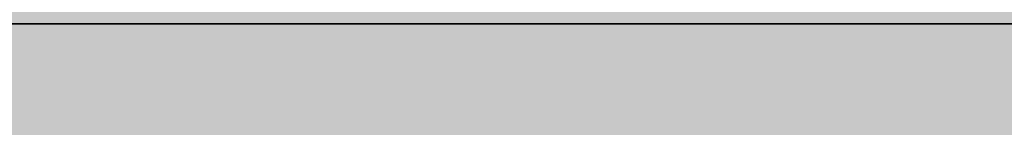
# Model space of a CAD drawing. Units: millimetres. Extents: x -22994 to 29398, y -19990 to 20176.
# Tile 72 of 135: x 226.355 to 227.437, y 83.446 to 83.564. Entities that reach past the tile are written whole.
import ezdxf
from ezdxf import colors
from ezdxf.entities.mleader import LeaderData, LeaderLine
from ezdxf.math import Vec2, Vec3

# ---------------------------------------------------------------- set-up
doc = ezdxf.new("R2010")
doc.units = ezdxf.units.MM
doc.header["$MEASUREMENT"] = 0
for name, color, linetype, lineweight in [('M-ANNO-TEXT', 7, 'Continuous', 25), ('M-DIMS', 2, 'Continuous', 18), ('M-EQPM-PATT', 7, 'Continuous', 18), ('M-PIPE', 7, 'Continuous', 35)]:
    doc.layers.add(name, color=color, linetype=linetype, lineweight=lineweight)
doc.styles.get("Standard").update_dxf_attribs({"font": 'arial.ttf'})
doc.dimstyles.get("Standard").update_dxf_attribs({"dimtxt": 0.18, "dimasz": 10000, "dimexe": 0.18, "dimexo": 0.0625, "dimgap": 0.09, "dimtad": 0, "dimtih": 1, "dimtoh": 1, "dimdec": 0, "dimzin": 0, "dimdsep": 46, "dimtxsty": 'Standard', "dimcen": 0.09, "dimadec": 0, "dimazin": 0, "dimtfac": 1, "dimtdec": 0, "dimtofl": 0, "dimtmove": 0, "dimatfit": 3, "dimfxl": 1, "dimtolj": 1, "dimtzin": 0, "dimlwd": 30, "dimarcsym": 0})

# ---------------------------------------------------------------- blocks, each defined once
blk = doc.blocks.new('*D2')
at = {"layer": 'Defpoints', "color": 0, "transparency": 16777216}
for p in [(6.6773, 10.2713), (290.852, 10.2713), (290.852, -5.0787)]:
    blk.add_point(p, dxfattribs=at)
at = {"layer": 'M-DIMS', "color": 0, "lineweight": -2, "transparency": 16777216}
for p, q in [((6.6773, 10.2088), (6.6773, -5.2587)), ((290.852, 10.2088), (290.852, -5.2587))]:
    blk.add_line(p, q, dxfattribs=at)
at = {"layer": 'M-DIMS', "color": 0, "lineweight": 30, "transparency": 16777216}
for p, q in [((-9993.3227, -5.0787), (-19993.3227, -5.0787)), ((10290.852, -5.0787), (20290.852, -5.0787))]:
    blk.add_line(p, q, dxfattribs=at)
at = {"layer": 'M-DIMS', "color": 0, "transparency": 16777216}
for points in [[(-9993.3227, 1661.5879), (-9993.3227, -1671.7454), (6.6773, -5.0787)], [(10290.852, 1661.5879), (10290.852, -1671.7454), (290.852, -5.0787)]]:
    blk.add_solid(points, dxfattribs=at)
at = {"layer": 'M-DIMS', "color": 0, "transparency": 16777216, "insert": (148.7647, -5.0787), "char_height": 0.18, "attachment_point": 5}
blk.add_mtext('\\A1;284.2', dxfattribs=at)
blk = doc.blocks.new('*D3')
at = {"layer": 'Defpoints', "color": 0, "transparency": 16777216}
for p in [(110.2647, 204.1654), (110.2647, 176.3662), (95.8327, 127.967)]:
    blk.add_point(p, dxfattribs=at)
at = {"layer": 'M-DIMS', "color": 0, "lineweight": -2, "transparency": 16777216}
for p, q in [((95.8327, 128.0295), (95.8327, 204.3454)), ((110.2647, 176.4287), (110.2647, 204.3454))]:
    blk.add_line(p, q, dxfattribs=at)
at = {"layer": 'M-DIMS', "color": 0, "lineweight": 30, "transparency": 16777216}
for p, q in [((-9904.1673, 204.1654), (-19904.1673, 204.1654)), ((10110.2647, 204.1654), (20110.2647, 204.1654))]:
    blk.add_line(p, q, dxfattribs=at)
at = {"layer": 'M-DIMS', "color": 0, "transparency": 16777216}
for points in [[(-9904.1673, 1870.8321), (-9904.1673, -1462.5013), (95.8327, 204.1654)], [(10110.2647, 1870.8321), (10110.2647, -1462.5013), (110.2647, 204.1654)]]:
    blk.add_solid(points, dxfattribs=at)
at = {"layer": 'M-DIMS', "color": 0, "transparency": 16777216, "insert": (103.0487, 204.1654), "char_height": 0.18, "attachment_point": 5}
blk.add_mtext('\\A1;14.432', dxfattribs=at)
blk = doc.blocks.new('*D4')
at = {"layer": 'Defpoints', "color": 0, "transparency": 16777216}
for p in [(116.2647, 204.1654), (110.2647, 176.3662), (116.2647, 176.3662)]:
    blk.add_point(p, dxfattribs=at)
at = {"layer": 'M-DIMS', "color": 0, "lineweight": -2, "transparency": 16777216}
for p, q in [((110.2647, 176.4287), (110.2647, 204.3454)), ((116.2647, 176.4287), (116.2647, 204.3454))]:
    blk.add_line(p, q, dxfattribs=at)
at = {"layer": 'M-DIMS', "color": 0, "lineweight": 30, "transparency": 16777216}
for p, q in [((-9889.7353, 204.1654), (-19889.7353, 204.1654)), ((10116.2647, 204.1654), (20116.2647, 204.1654))]:
    blk.add_line(p, q, dxfattribs=at)
at = {"layer": 'M-DIMS', "color": 0, "transparency": 16777216}
for points in [[(-9889.7353, 1870.8321), (-9889.7353, -1462.5013), (110.2647, 204.1654)], [(10116.2647, 1870.8321), (10116.2647, -1462.5013), (116.2647, 204.1654)]]:
    blk.add_solid(points, dxfattribs=at)
at = {"layer": 'M-DIMS', "color": 0, "transparency": 16777216, "insert": (113.2647, 204.1654), "char_height": 0.18, "attachment_point": 5}
blk.add_mtext('\\A1;6', dxfattribs=at)
blk = doc.blocks.new('*D5')
at = {"layer": 'Defpoints', "color": 0, "transparency": 16777216}
for p in [(181.2647, 204.1654), (116.2647, 176.3662), (181.2647, 176.3662)]:
    blk.add_point(p, dxfattribs=at)
at = {"layer": 'M-DIMS', "color": 0, "lineweight": -2, "transparency": 16777216}
for p, q in [((116.2647, 176.4287), (116.2647, 204.3454)), ((181.2647, 176.4287), (181.2647, 204.3454))]:
    blk.add_line(p, q, dxfattribs=at)
at = {"layer": 'M-DIMS', "color": 0, "lineweight": 30, "transparency": 16777216}
for p, q in [((-9883.7353, 204.1654), (-19883.7353, 204.1654)), ((10181.2647, 204.1654), (20181.2647, 204.1654))]:
    blk.add_line(p, q, dxfattribs=at)
at = {"layer": 'M-DIMS', "color": 0, "transparency": 16777216}
for points in [[(-9883.7353, 1870.8321), (-9883.7353, -1462.5013), (116.2647, 204.1654)], [(10181.2647, 1870.8321), (10181.2647, -1462.5013), (181.2647, 204.1654)]]:
    blk.add_solid(points, dxfattribs=at)
at = {"layer": 'M-DIMS', "color": 0, "transparency": 16777216, "insert": (148.7647, 204.1654), "char_height": 0.18, "attachment_point": 5}
blk.add_mtext('\\A1;65', dxfattribs=at)
blk = doc.blocks.new('*D6')
at = {"layer": 'Defpoints', "color": 0, "transparency": 16777216}
for p in [(187.2647, 204.1654), (181.2647, 176.3662), (187.2647, 176.3662)]:
    blk.add_point(p, dxfattribs=at)
at = {"layer": 'M-DIMS', "color": 0, "lineweight": -2, "transparency": 16777216}
for p, q in [((181.2647, 176.4287), (181.2647, 204.3454)), ((187.2647, 176.4287), (187.2647, 204.3454))]:
    blk.add_line(p, q, dxfattribs=at)
at = {"layer": 'M-DIMS', "color": 0, "lineweight": 30, "transparency": 16777216}
for p, q in [((-9818.7353, 204.1654), (-19818.7353, 204.1654)), ((10187.2647, 204.1654), (20187.2647, 204.1654))]:
    blk.add_line(p, q, dxfattribs=at)
at = {"layer": 'M-DIMS', "color": 0, "transparency": 16777216}
for points in [[(-9818.7353, 1870.8321), (-9818.7353, -1462.5013), (181.2647, 204.1654)], [(10187.2647, 1870.8321), (10187.2647, -1462.5013), (187.2647, 204.1654)]]:
    blk.add_solid(points, dxfattribs=at)
at = {"layer": 'M-DIMS', "color": 0, "transparency": 16777216, "insert": (184.2647, 204.1654), "char_height": 0.18, "attachment_point": 5}
blk.add_mtext('\\A1;6', dxfattribs=at)
blk = doc.blocks.new('*D7')
at = {"layer": 'Defpoints', "color": 0, "transparency": 16777216}
for p in [(201.6967, 204.1654), (187.2647, 176.3662), (201.6967, 127.967)]:
    blk.add_point(p, dxfattribs=at)
at = {"layer": 'M-DIMS', "color": 0, "lineweight": -2, "transparency": 16777216}
for p, q in [((187.2647, 176.4287), (187.2647, 204.3454)), ((201.6967, 128.0295), (201.6967, 204.3454))]:
    blk.add_line(p, q, dxfattribs=at)
at = {"layer": 'M-DIMS', "color": 0, "lineweight": 30, "transparency": 16777216}
for p, q in [((-9812.7353, 204.1654), (-19812.7353, 204.1654)), ((10201.6967, 204.1654), (20201.6967, 204.1654))]:
    blk.add_line(p, q, dxfattribs=at)
at = {"layer": 'M-DIMS', "color": 0, "transparency": 16777216}
for points in [[(-9812.7353, 1870.8321), (-9812.7353, -1462.5013), (187.2647, 204.1654)], [(10201.6967, 1870.8321), (10201.6967, -1462.5013), (201.6967, 204.1654)]]:
    blk.add_solid(points, dxfattribs=at)
at = {"layer": 'M-DIMS', "color": 0, "transparency": 16777216, "insert": (194.4807, 204.1654), "char_height": 0.18, "attachment_point": 5}
blk.add_mtext('\\A1;14.432', dxfattribs=at)
blk = doc.blocks.new('*D8')
at = {"layer": 'Defpoints', "color": 0, "transparency": 16777216}
for p in [(227.6485, 204.1654), (227.6485, 146.7296), (201.6967, 127.967)]:
    blk.add_point(p, dxfattribs=at)
at = {"layer": 'M-DIMS', "color": 0, "lineweight": -2, "transparency": 16777216}
for p, q in [((201.6967, 128.0295), (201.6967, 204.3454)), ((227.6485, 146.7921), (227.6485, 204.3454))]:
    blk.add_line(p, q, dxfattribs=at)
at = {"layer": 'M-DIMS', "color": 0, "lineweight": 30, "transparency": 16777216}
for p, q in [((-9798.3033, 204.1654), (-19798.3033, 204.1654)), ((10227.6485, 204.1654), (20227.6485, 204.1654))]:
    blk.add_line(p, q, dxfattribs=at)
at = {"layer": 'M-DIMS', "color": 0, "transparency": 16777216}
for points in [[(-9798.3033, 1870.8321), (-9798.3033, -1462.5013), (201.6967, 204.1654)], [(10227.6485, 1870.8321), (10227.6485, -1462.5013), (227.6485, 204.1654)]]:
    blk.add_solid(points, dxfattribs=at)
at = {"layer": 'M-DIMS', "color": 0, "transparency": 16777216, "insert": (214.6726, 204.1654), "char_height": 0.18, "attachment_point": 5}
blk.add_mtext('\\A1;25.95', dxfattribs=at)
blk = doc.blocks.new('*D9')
at = {"layer": 'Defpoints', "color": 0, "transparency": 16777216}
for p in [(187.2647, 176.3662), (306.202, 176.3662), (290.852, 10.2713)]:
    blk.add_point(p, dxfattribs=at)
at = {"layer": 'M-DIMS', "color": 0, "lineweight": 30, "transparency": 16777216}
for p, q in [((306.202, 10176.3662), (306.202, 20176.3662)), ((306.202, -9989.7287), (306.202, -19989.7287))]:
    blk.add_line(p, q, dxfattribs=at)
at = {"layer": 'M-DIMS', "color": 0, "lineweight": -2, "transparency": 16777216}
for p, q in [((187.3272, 176.3662), (306.382, 176.3662)), ((290.9145, 10.2713), (306.382, 10.2713))]:
    blk.add_line(p, q, dxfattribs=at)
at = {"layer": 'M-DIMS', "color": 0, "transparency": 16777216}
for points in [[(-1360.4646, 10176.3662), (1972.8687, 10176.3662), (306.202, 176.3662)], [(-1360.4646, -9989.7287), (1972.8687, -9989.7287), (306.202, 10.2713)]]:
    blk.add_solid(points, dxfattribs=at)
at = {"layer": 'M-DIMS', "color": 0, "transparency": 16777216, "insert": (306.202, 93.3187), "char_height": 0.18, "attachment_point": 5}
blk.add_mtext('\\A1;166.1', dxfattribs=at)
blk = doc.blocks.new('*D10')
at = {"layer": 'Defpoints', "color": 0, "transparency": 16777216}
for p in [(125.6498, 136.0713), (133.3459, 136.0713), (133.3459, -5.0787)]:
    blk.add_point(p, dxfattribs=at)
at = {"layer": 'M-DIMS', "color": 0, "lineweight": -2, "transparency": 16777216}
for p, q in [((125.6498, 136.0088), (125.6498, -5.2587)), ((133.3459, 136.0088), (133.3459, -5.2587))]:
    blk.add_line(p, q, dxfattribs=at)
at = {"layer": 'M-DIMS', "color": 0, "lineweight": 30, "transparency": 16777216}
for p, q in [((-9874.3502, -5.0787), (-19874.3502, -5.0787)), ((10133.3459, -5.0787), (20133.3459, -5.0787))]:
    blk.add_line(p, q, dxfattribs=at)
at = {"layer": 'M-DIMS', "color": 0, "transparency": 16777216}
for points in [[(-9874.3502, 1661.5879), (-9874.3502, -1671.7454), (125.6498, -5.0787)], [(10133.3459, 1661.5879), (10133.3459, -1671.7454), (133.3459, -5.0787)]]:
    blk.add_solid(points, dxfattribs=at)
at = {"layer": 'M-DIMS', "color": 0, "transparency": 16777216, "insert": (129.4978, -5.0787), "char_height": 0.18, "attachment_point": 5}
blk.add_mtext('\\A1;7.696', dxfattribs=at)
blk = doc.blocks.new('*D11')
at = {"layer": 'Defpoints', "color": 0, "transparency": 16777216}
for p in [(133.3459, 136.0713), (135.6498, 136.0713), (135.6498, -5.0787)]:
    blk.add_point(p, dxfattribs=at)
at = {"layer": 'M-DIMS', "color": 0, "lineweight": -2, "transparency": 16777216}
for p, q in [((133.3459, 136.0088), (133.3459, -5.2587)), ((135.6498, 136.0088), (135.6498, -5.2587))]:
    blk.add_line(p, q, dxfattribs=at)
at = {"layer": 'M-DIMS', "color": 0, "lineweight": 30, "transparency": 16777216}
for p, q in [((-9866.6541, -5.0787), (-19866.6541, -5.0787)), ((10135.6498, -5.0787), (20135.6498, -5.0787))]:
    blk.add_line(p, q, dxfattribs=at)
at = {"layer": 'M-DIMS', "color": 0, "transparency": 16777216}
for points in [[(-9866.6541, 1661.5879), (-9866.6541, -1671.7454), (133.3459, -5.0787)], [(10135.6498, 1661.5879), (10135.6498, -1671.7454), (135.6498, -5.0787)]]:
    blk.add_solid(points, dxfattribs=at)
at = {"layer": 'M-DIMS', "color": 0, "transparency": 16777216, "insert": (134.4978, -5.0787), "char_height": 0.18, "attachment_point": 5}
blk.add_mtext('\\A1;2.304', dxfattribs=at)
blk = doc.blocks.new('*D12')
at = {"layer": 'Defpoints', "color": 0, "transparency": 16777216}
for p in [(135.6498, 136.0713), (145.6498, 136.0713), (145.6498, -5.0787)]:
    blk.add_point(p, dxfattribs=at)
at = {"layer": 'M-DIMS', "color": 0, "lineweight": -2, "transparency": 16777216}
for p, q in [((135.6498, 136.0088), (135.6498, -5.2587)), ((145.6498, 136.0088), (145.6498, -5.2587))]:
    blk.add_line(p, q, dxfattribs=at)
at = {"layer": 'M-DIMS', "color": 0, "lineweight": 30, "transparency": 16777216}
for p, q in [((-9864.3502, -5.0787), (-19864.3502, -5.0787)), ((10145.6498, -5.0787), (20145.6498, -5.0787))]:
    blk.add_line(p, q, dxfattribs=at)
at = {"layer": 'M-DIMS', "color": 0, "transparency": 16777216}
for points in [[(-9864.3502, 1661.5879), (-9864.3502, -1671.7454), (135.6498, -5.0787)], [(10145.6498, 1661.5879), (10145.6498, -1671.7454), (145.6498, -5.0787)]]:
    blk.add_solid(points, dxfattribs=at)
at = {"layer": 'M-DIMS', "color": 0, "transparency": 16777216, "insert": (140.6498, -5.0787), "char_height": 0.18, "attachment_point": 5}
blk.add_mtext('\\A1;10', dxfattribs=at)
blk = doc.blocks.new('*D13')
at = {"layer": 'Defpoints', "color": 0, "transparency": 16777216}
for p in [(145.6498, 136.0713), (155.6498, 136.0713), (155.6498, -5.0787)]:
    blk.add_point(p, dxfattribs=at)
at = {"layer": 'M-DIMS', "color": 0, "lineweight": -2, "transparency": 16777216}
for p, q in [((145.6498, 136.0088), (145.6498, -5.2587)), ((155.6498, 136.0088), (155.6498, -5.2587))]:
    blk.add_line(p, q, dxfattribs=at)
at = {"layer": 'M-DIMS', "color": 0, "lineweight": 30, "transparency": 16777216}
for p, q in [((-9854.3502, -5.0787), (-19854.3502, -5.0787)), ((10155.6498, -5.0787), (20155.6498, -5.0787))]:
    blk.add_line(p, q, dxfattribs=at)
at = {"layer": 'M-DIMS', "color": 0, "transparency": 16777216}
for points in [[(-9854.3502, 1661.5879), (-9854.3502, -1671.7454), (145.6498, -5.0787)], [(10155.6498, 1661.5879), (10155.6498, -1671.7454), (155.6498, -5.0787)]]:
    blk.add_solid(points, dxfattribs=at)
at = {"layer": 'M-DIMS', "color": 0, "transparency": 16777216, "insert": (150.6498, -5.0787), "char_height": 0.18, "attachment_point": 5}
blk.add_mtext('\\A1;10', dxfattribs=at)
blk = doc.blocks.new('*D14')
at = {"layer": 'Defpoints', "color": 0, "transparency": 16777216}
for p in [(155.6498, 136.0713), (165.6498, 136.0713), (165.6498, -5.0787)]:
    blk.add_point(p, dxfattribs=at)
at = {"layer": 'M-DIMS', "color": 0, "lineweight": -2, "transparency": 16777216}
for p, q in [((155.6498, 136.0088), (155.6498, -5.2587)), ((165.6498, 136.0088), (165.6498, -5.2587))]:
    blk.add_line(p, q, dxfattribs=at)
at = {"layer": 'M-DIMS', "color": 0, "lineweight": 30, "transparency": 16777216}
for p, q in [((-9844.3502, -5.0787), (-19844.3502, -5.0787)), ((10165.6498, -5.0787), (20165.6498, -5.0787))]:
    blk.add_line(p, q, dxfattribs=at)
at = {"layer": 'M-DIMS', "color": 0, "transparency": 16777216}
for points in [[(-9844.3502, 1661.5879), (-9844.3502, -1671.7454), (155.6498, -5.0787)], [(10165.6498, 1661.5879), (10165.6498, -1671.7454), (165.6498, -5.0787)]]:
    blk.add_solid(points, dxfattribs=at)
at = {"layer": 'M-DIMS', "color": 0, "transparency": 16777216, "insert": (160.6498, -5.0787), "char_height": 0.18, "attachment_point": 5}
blk.add_mtext('\\A1;10', dxfattribs=at)
blk = doc.blocks.new('*D15')
at = {"layer": 'Defpoints', "color": 0, "transparency": 16777216}
for p in [(173.3459, 154.788), (173.3459, 136.0713), (306.202, 136.0713)]:
    blk.add_point(p, dxfattribs=at)
at = {"layer": 'M-DIMS', "color": 0, "lineweight": 30, "transparency": 16777216}
for p, q in [((306.202, 10154.788), (306.202, 20154.788)), ((306.202, -9863.9287), (306.202, -19863.9287))]:
    blk.add_line(p, q, dxfattribs=at)
at = {"layer": 'M-DIMS', "color": 0, "lineweight": -2, "transparency": 16777216}
for p, q in [((173.4084, 154.788), (306.382, 154.788)), ((173.4084, 136.0713), (306.382, 136.0713))]:
    blk.add_line(p, q, dxfattribs=at)
at = {"layer": 'M-DIMS', "color": 0, "transparency": 16777216}
for points in [[(-1360.4646, 10154.788), (1972.8687, 10154.788), (306.202, 154.788)], [(-1360.4646, -9863.9287), (1972.8687, -9863.9287), (306.202, 136.0713)]]:
    blk.add_solid(points, dxfattribs=at)
at = {"layer": 'M-DIMS', "color": 0, "transparency": 16777216, "insert": (306.202, 145.4297), "char_height": 0.18, "attachment_point": 5}
blk.add_mtext('\\A1;18.717', dxfattribs=at)
blk = doc.blocks.new('*D16')
at = {"layer": 'Defpoints', "color": 0, "transparency": 16777216}
for p in [(120.1702, 204.1654), (110.4658, 48.0349), (120.1702, 48.0349)]:
    blk.add_point(p, dxfattribs=at)
at = {"layer": 'M-DIMS', "color": 0, "lineweight": -2, "transparency": 16777216}
for p, q in [((110.4658, 48.0974), (110.4658, 204.3454)), ((120.1702, 48.0974), (120.1702, 204.3454))]:
    blk.add_line(p, q, dxfattribs=at)
at = {"layer": 'M-DIMS', "color": 0, "lineweight": 30, "transparency": 16777216}
for p, q in [((-9889.5342, 204.1654), (-19889.5342, 204.1654)), ((10120.1702, 204.1654), (20120.1702, 204.1654))]:
    blk.add_line(p, q, dxfattribs=at)
at = {"layer": 'M-DIMS', "color": 0, "transparency": 16777216}
for points in [[(-9889.5342, 1870.8321), (-9889.5342, -1462.5013), (110.4658, 204.1654)], [(10120.1702, 1870.8321), (10120.1702, -1462.5013), (120.1702, 204.1654)]]:
    blk.add_solid(points, dxfattribs=at)
at = {"layer": 'M-DIMS', "color": 0, "transparency": 16777216, "insert": (115.318, 204.1654), "char_height": 0.18, "attachment_point": 5}
blk.add_mtext('\\A1;9.704', dxfattribs=at)
blk = doc.blocks.new('*D17')
at = {"layer": 'Defpoints', "color": 0, "transparency": 16777216}
for p in [(126.1702, 204.1654), (120.1702, 48.0349), (126.1702, 48.0349)]:
    blk.add_point(p, dxfattribs=at)
at = {"layer": 'M-DIMS', "color": 0, "lineweight": -2, "transparency": 16777216}
for p, q in [((120.1702, 48.0974), (120.1702, 204.3454)), ((126.1702, 48.0974), (126.1702, 204.3454))]:
    blk.add_line(p, q, dxfattribs=at)
at = {"layer": 'M-DIMS', "color": 0, "lineweight": 30, "transparency": 16777216}
for p, q in [((-9879.8298, 204.1654), (-19879.8298, 204.1654)), ((10126.1702, 204.1654), (20126.1702, 204.1654))]:
    blk.add_line(p, q, dxfattribs=at)
at = {"layer": 'M-DIMS', "color": 0, "transparency": 16777216}
for points in [[(-9879.8298, 1870.8321), (-9879.8298, -1462.5013), (120.1702, 204.1654)], [(10126.1702, 1870.8321), (10126.1702, -1462.5013), (126.1702, 204.1654)]]:
    blk.add_solid(points, dxfattribs=at)
at = {"layer": 'M-DIMS', "color": 0, "transparency": 16777216, "insert": (123.1702, 204.1654), "char_height": 0.18, "attachment_point": 5}
blk.add_mtext('\\A1;6', dxfattribs=at)
blk = doc.blocks.new('*D18')
at = {"layer": 'Defpoints', "color": 0, "transparency": 16777216}
for p in [(132.1702, 204.1654), (126.1702, 48.0349), (132.1702, 48.0349)]:
    blk.add_point(p, dxfattribs=at)
at = {"layer": 'M-DIMS', "color": 0, "lineweight": -2, "transparency": 16777216}
for p, q in [((126.1702, 48.0974), (126.1702, 204.3454)), ((132.1702, 48.0974), (132.1702, 204.3454))]:
    blk.add_line(p, q, dxfattribs=at)
at = {"layer": 'M-DIMS', "color": 0, "lineweight": 30, "transparency": 16777216}
for p, q in [((-9873.8298, 204.1654), (-19873.8298, 204.1654)), ((10132.1702, 204.1654), (20132.1702, 204.1654))]:
    blk.add_line(p, q, dxfattribs=at)
at = {"layer": 'M-DIMS', "color": 0, "transparency": 16777216}
for points in [[(-9873.8298, 1870.8321), (-9873.8298, -1462.5013), (126.1702, 204.1654)], [(10132.1702, 1870.8321), (10132.1702, -1462.5013), (132.1702, 204.1654)]]:
    blk.add_solid(points, dxfattribs=at)
at = {"layer": 'M-DIMS', "color": 0, "transparency": 16777216, "insert": (129.1702, 204.1654), "char_height": 0.18, "attachment_point": 5}
blk.add_mtext('\\A1;6', dxfattribs=at)
blk = doc.blocks.new('*D19')
at = {"layer": 'Defpoints', "color": 0, "transparency": 16777216}
for p in [(138.1702, 204.1654), (132.1702, 48.0349), (138.1702, 48.0349)]:
    blk.add_point(p, dxfattribs=at)
at = {"layer": 'M-DIMS', "color": 0, "lineweight": -2, "transparency": 16777216}
for p, q in [((132.1702, 48.0974), (132.1702, 204.3454)), ((138.1702, 48.0974), (138.1702, 204.3454))]:
    blk.add_line(p, q, dxfattribs=at)
at = {"layer": 'M-DIMS', "color": 0, "lineweight": 30, "transparency": 16777216}
for p, q in [((-9867.8298, 204.1654), (-19867.8298, 204.1654)), ((10138.1702, 204.1654), (20138.1702, 204.1654))]:
    blk.add_line(p, q, dxfattribs=at)
at = {"layer": 'M-DIMS', "color": 0, "transparency": 16777216}
for points in [[(-9867.8298, 1870.8321), (-9867.8298, -1462.5013), (132.1702, 204.1654)], [(10138.1702, 1870.8321), (10138.1702, -1462.5013), (138.1702, 204.1654)]]:
    blk.add_solid(points, dxfattribs=at)
at = {"layer": 'M-DIMS', "color": 0, "transparency": 16777216, "insert": (135.1702, 204.1654), "char_height": 0.18, "attachment_point": 5}
blk.add_mtext('\\A1;6', dxfattribs=at)
blk = doc.blocks.new('*D20')
at = {"layer": 'Defpoints', "color": 0, "transparency": 16777216}
for p in [(144.1702, 204.1654), (138.1702, 48.0349), (144.1702, 48.0349)]:
    blk.add_point(p, dxfattribs=at)
at = {"layer": 'M-DIMS', "color": 0, "lineweight": -2, "transparency": 16777216}
for p, q in [((138.1702, 48.0974), (138.1702, 204.3454)), ((144.1702, 48.0974), (144.1702, 204.3454))]:
    blk.add_line(p, q, dxfattribs=at)
at = {"layer": 'M-DIMS', "color": 0, "lineweight": 30, "transparency": 16777216}
for p, q in [((-9861.8298, 204.1654), (-19861.8298, 204.1654)), ((10144.1702, 204.1654), (20144.1702, 204.1654))]:
    blk.add_line(p, q, dxfattribs=at)
at = {"layer": 'M-DIMS', "color": 0, "transparency": 16777216}
for points in [[(-9861.8298, 1870.8321), (-9861.8298, -1462.5013), (138.1702, 204.1654)], [(10144.1702, 1870.8321), (10144.1702, -1462.5013), (144.1702, 204.1654)]]:
    blk.add_solid(points, dxfattribs=at)
at = {"layer": 'M-DIMS', "color": 0, "transparency": 16777216, "insert": (141.1702, 204.1654), "char_height": 0.18, "attachment_point": 5}
blk.add_mtext('\\A1;6', dxfattribs=at)
blk = doc.blocks.new('*D21')
at = {"layer": 'Defpoints', "color": 0, "transparency": 16777216}
for p in [(149.1157, 204.1654), (144.1702, 48.0349), (149.1157, 48.0349)]:
    blk.add_point(p, dxfattribs=at)
at = {"layer": 'M-DIMS', "color": 0, "lineweight": -2, "transparency": 16777216}
for p, q in [((144.1702, 48.0974), (144.1702, 204.3454)), ((149.1157, 48.0974), (149.1157, 204.3454))]:
    blk.add_line(p, q, dxfattribs=at)
at = {"layer": 'M-DIMS', "color": 0, "lineweight": 30, "transparency": 16777216}
for p, q in [((-9855.8298, 204.1654), (-19855.8298, 204.1654)), ((10149.1157, 204.1654), (20149.1157, 204.1654))]:
    blk.add_line(p, q, dxfattribs=at)
at = {"layer": 'M-DIMS', "color": 0, "transparency": 16777216}
for points in [[(-9855.8298, 1870.8321), (-9855.8298, -1462.5013), (144.1702, 204.1654)], [(10149.1157, 1870.8321), (10149.1157, -1462.5013), (149.1157, 204.1654)]]:
    blk.add_solid(points, dxfattribs=at)
at = {"layer": 'M-DIMS', "color": 0, "transparency": 16777216, "insert": (146.6429, 204.1654), "char_height": 0.18, "attachment_point": 5}
blk.add_mtext('\\A1;4.945', dxfattribs=at)
blk = doc.blocks.new('*D22')
at = {"layer": 'Defpoints', "color": 0, "transparency": 16777216}
for p in [(149.1157, 30.9895), (155.1157, 30.9895), (155.1157, -5.0787)]:
    blk.add_point(p, dxfattribs=at)
at = {"layer": 'M-DIMS', "color": 0, "lineweight": -2, "transparency": 16777216}
for p, q in [((149.1157, 30.927), (149.1157, -5.2587)), ((155.1157, 30.927), (155.1157, -5.2587))]:
    blk.add_line(p, q, dxfattribs=at)
at = {"layer": 'M-DIMS', "color": 0, "lineweight": 30, "transparency": 16777216}
for p, q in [((-9850.8843, -5.0787), (-19850.8843, -5.0787)), ((10155.1157, -5.0787), (20155.1157, -5.0787))]:
    blk.add_line(p, q, dxfattribs=at)
at = {"layer": 'M-DIMS', "color": 0, "transparency": 16777216}
for points in [[(-9850.8843, 1661.5879), (-9850.8843, -1671.7454), (149.1157, -5.0787)], [(10155.1157, 1661.5879), (10155.1157, -1671.7454), (155.1157, -5.0787)]]:
    blk.add_solid(points, dxfattribs=at)
at = {"layer": 'M-DIMS', "color": 0, "transparency": 16777216, "insert": (152.1157, -5.0787), "char_height": 0.18, "attachment_point": 5}
blk.add_mtext('\\A1;6', dxfattribs=at)
blk = doc.blocks.new('*D23')
at = {"layer": 'Defpoints', "color": 0, "transparency": 16777216}
for p in [(155.1157, 30.9895), (161.1157, 30.9895), (161.1157, -5.0787)]:
    blk.add_point(p, dxfattribs=at)
at = {"layer": 'M-DIMS', "color": 0, "lineweight": -2, "transparency": 16777216}
for p, q in [((155.1157, 30.927), (155.1157, -5.2587)), ((161.1157, 30.927), (161.1157, -5.2587))]:
    blk.add_line(p, q, dxfattribs=at)
at = {"layer": 'M-DIMS', "color": 0, "lineweight": 30, "transparency": 16777216}
for p, q in [((-9844.8843, -5.0787), (-19844.8843, -5.0787)), ((10161.1157, -5.0787), (20161.1157, -5.0787))]:
    blk.add_line(p, q, dxfattribs=at)
at = {"layer": 'M-DIMS', "color": 0, "transparency": 16777216}
for points in [[(-9844.8843, 1661.5879), (-9844.8843, -1671.7454), (155.1157, -5.0787)], [(10161.1157, 1661.5879), (10161.1157, -1671.7454), (161.1157, -5.0787)]]:
    blk.add_solid(points, dxfattribs=at)
at = {"layer": 'M-DIMS', "color": 0, "transparency": 16777216, "insert": (158.1157, -5.0787), "char_height": 0.18, "attachment_point": 5}
blk.add_mtext('\\A1;6', dxfattribs=at)
blk = doc.blocks.new('*D24')
at = {"layer": 'Defpoints', "color": 0, "transparency": 16777216}
for p in [(161.1157, 30.9895), (166.4387, 30.9895), (166.4387, -5.0787)]:
    blk.add_point(p, dxfattribs=at)
at = {"layer": 'M-DIMS', "color": 0, "lineweight": -2, "transparency": 16777216}
for p, q in [((161.1157, 30.927), (161.1157, -5.2587)), ((166.4387, 30.927), (166.4387, -5.2587))]:
    blk.add_line(p, q, dxfattribs=at)
at = {"layer": 'M-DIMS', "color": 0, "lineweight": 30, "transparency": 16777216}
for p, q in [((-9838.8843, -5.0787), (-19838.8843, -5.0787)), ((10166.4387, -5.0787), (20166.4387, -5.0787))]:
    blk.add_line(p, q, dxfattribs=at)
at = {"layer": 'M-DIMS', "color": 0, "transparency": 16777216}
for points in [[(-9838.8843, 1661.5879), (-9838.8843, -1671.7454), (161.1157, -5.0787)], [(10166.4387, 1661.5879), (10166.4387, -1671.7454), (166.4387, -5.0787)]]:
    blk.add_solid(points, dxfattribs=at)
at = {"layer": 'M-DIMS', "color": 0, "transparency": 16777216, "insert": (163.7772, -5.0787), "char_height": 0.18, "attachment_point": 5}
blk.add_mtext('\\A1;5.323', dxfattribs=at)
blk = doc.blocks.new('*D25')
at = {"layer": 'Defpoints', "color": 0, "transparency": 16777216}
for p in [(166.4387, 30.9895), (172.4387, 30.9895), (172.4387, -5.0787)]:
    blk.add_point(p, dxfattribs=at)
at = {"layer": 'M-DIMS', "color": 0, "lineweight": -2, "transparency": 16777216}
for p, q in [((166.4387, 30.927), (166.4387, -5.2587)), ((172.4387, 30.927), (172.4387, -5.2587))]:
    blk.add_line(p, q, dxfattribs=at)
at = {"layer": 'M-DIMS', "color": 0, "lineweight": 30, "transparency": 16777216}
for p, q in [((-9833.5613, -5.0787), (-19833.5613, -5.0787)), ((10172.4387, -5.0787), (20172.4387, -5.0787))]:
    blk.add_line(p, q, dxfattribs=at)
at = {"layer": 'M-DIMS', "color": 0, "transparency": 16777216}
for points in [[(-9833.5613, 1661.5879), (-9833.5613, -1671.7454), (166.4387, -5.0787)], [(10172.4387, 1661.5879), (10172.4387, -1671.7454), (172.4387, -5.0787)]]:
    blk.add_solid(points, dxfattribs=at)
at = {"layer": 'M-DIMS', "color": 0, "transparency": 16777216, "insert": (169.4387, -5.0787), "char_height": 0.18, "attachment_point": 5}
blk.add_mtext('\\A1;6', dxfattribs=at)
blk = doc.blocks.new('*D26')
at = {"layer": 'Defpoints', "color": 0, "transparency": 16777216}
for p in [(172.4387, 30.9895), (178.4387, 30.9895), (178.4387, -5.0787)]:
    blk.add_point(p, dxfattribs=at)
at = {"layer": 'M-DIMS', "color": 0, "lineweight": -2, "transparency": 16777216}
for p, q in [((172.4387, 30.927), (172.4387, -5.2587)), ((178.4387, 30.927), (178.4387, -5.2587))]:
    blk.add_line(p, q, dxfattribs=at)
at = {"layer": 'M-DIMS', "color": 0, "lineweight": 30, "transparency": 16777216}
for p, q in [((-9827.5613, -5.0787), (-19827.5613, -5.0787)), ((10178.4387, -5.0787), (20178.4387, -5.0787))]:
    blk.add_line(p, q, dxfattribs=at)
at = {"layer": 'M-DIMS', "color": 0, "transparency": 16777216}
for points in [[(-9827.5613, 1661.5879), (-9827.5613, -1671.7454), (172.4387, -5.0787)], [(10178.4387, 1661.5879), (10178.4387, -1671.7454), (178.4387, -5.0787)]]:
    blk.add_solid(points, dxfattribs=at)
at = {"layer": 'M-DIMS', "color": 0, "transparency": 16777216, "insert": (175.4387, -5.0787), "char_height": 0.18, "attachment_point": 5}
blk.add_mtext('\\A1;6', dxfattribs=at)
blk = doc.blocks.new('*D27')
at = {"layer": 'Defpoints', "color": 0, "transparency": 16777216}
for p in [(178.4387, 30.9895), (188.1175, 30.9895), (188.1175, -5.0787)]:
    blk.add_point(p, dxfattribs=at)
at = {"layer": 'M-DIMS', "color": 0, "lineweight": -2, "transparency": 16777216}
for p, q in [((178.4387, 30.927), (178.4387, -5.2587)), ((188.1175, 30.927), (188.1175, -5.2587))]:
    blk.add_line(p, q, dxfattribs=at)
at = {"layer": 'M-DIMS', "color": 0, "lineweight": 30, "transparency": 16777216}
for p, q in [((-9821.5613, -5.0787), (-19821.5613, -5.0787)), ((10188.1175, -5.0787), (20188.1175, -5.0787))]:
    blk.add_line(p, q, dxfattribs=at)
at = {"layer": 'M-DIMS', "color": 0, "transparency": 16777216}
for points in [[(-9821.5613, 1661.5879), (-9821.5613, -1671.7454), (178.4387, -5.0787)], [(10188.1175, 1661.5879), (10188.1175, -1671.7454), (188.1175, -5.0787)]]:
    blk.add_solid(points, dxfattribs=at)
at = {"layer": 'M-DIMS', "color": 0, "transparency": 16777216, "insert": (183.2781, -5.0787), "char_height": 0.18, "attachment_point": 5}
blk.add_mtext('\\A1;9.679', dxfattribs=at)
blk = doc.blocks.new('*D28')
at = {"layer": 'Defpoints', "color": 0, "transparency": 16777216}
for p in [(188.1175, 48.0349), (306.202, 48.0349), (188.1175, 30.9895)]:
    blk.add_point(p, dxfattribs=at)
at = {"layer": 'M-DIMS', "color": 0, "lineweight": 30, "transparency": 16777216}
for p, q in [((306.202, 10048.0349), (306.202, 20048.0349)), ((306.202, -9969.0105), (306.202, -19969.0105))]:
    blk.add_line(p, q, dxfattribs=at)
at = {"layer": 'M-DIMS', "color": 0, "lineweight": -2, "transparency": 16777216}
for p, q in [((188.18, 48.0349), (306.382, 48.0349)), ((188.18, 30.9895), (306.382, 30.9895))]:
    blk.add_line(p, q, dxfattribs=at)
at = {"layer": 'M-DIMS', "color": 0, "transparency": 16777216}
for points in [[(-1360.4646, 10048.0349), (1972.8687, 10048.0349), (306.202, 48.0349)], [(-1360.4646, -9969.0105), (1972.8687, -9969.0105), (306.202, 30.9895)]]:
    blk.add_solid(points, dxfattribs=at)
at = {"layer": 'M-DIMS', "color": 0, "transparency": 16777216, "insert": (306.202, 39.5122), "char_height": 0.18, "attachment_point": 5}
blk.add_mtext('\\A1;17.045', dxfattribs=at)
blk = doc.blocks.new('*D29')
at = {"layer": 'Defpoints', "color": 0, "transparency": 16777216}
for p in [(36.8006, 80.045), (64.0296, 80.045)]:
    blk.add_point(p, dxfattribs=at)
at = {"layer": 'M-DIMS', "color": 0, "lineweight": -2, "transparency": 16777216}
for p, q in [((50.4151, 79.955), (50.4151, 80.135)), ((50.3251, 80.045), (50.5051, 80.045))]:
    blk.add_line(p, q, dxfattribs=at)
at = {"layer": 'M-DIMS', "color": 0, "lineweight": 30, "transparency": 16777216}
blk.add_line((20064.0296, 80.0303), (10064.0296, 80.0377), dxfattribs=at)
at = {"layer": 'M-DIMS', "color": 0, "transparency": 16777216}
blk.add_solid([(10064.0309, 1746.7043), (10064.0284, -1586.629), (64.0296, 80.045)], dxfattribs=at)
at = {"layer": 'M-DIMS', "color": 0, "transparency": 16777216, "insert": (20064.5213, 80.0303), "char_height": 0.18, "attachment_point": 5}
blk.add_mtext('\\A1;∅27.23', dxfattribs=at)
blk = doc.blocks.new('*D30')
at = {"layer": 'Defpoints', "color": 0, "transparency": 16777216}
for p in [(216.3148, 146.7291), (238.9821, 146.73)]:
    blk.add_point(p, dxfattribs=at)
at = {"layer": 'M-DIMS', "color": 0, "lineweight": 30, "transparency": 16777216}
blk.add_line((20238.9821, 147.4959), (10238.9821, 147.1129), dxfattribs=at)
at = {"layer": 'M-DIMS', "color": 0, "lineweight": -2, "transparency": 16777216}
for p, q in [((227.6485, 146.6396), (227.6485, 146.8196)), ((227.5585, 146.7296), (227.7385, 146.7296))]:
    blk.add_line(p, q, dxfattribs=at)
at = {"layer": 'M-DIMS', "color": 0, "transparency": 16777216}
blk.add_solid([(10238.9183, 1813.7796), (10239.0459, -1519.5537), (238.9821, 146.73)], dxfattribs=at)
at = {"layer": 'M-DIMS', "color": 0, "transparency": 16777216, "insert": (20239.5436, 147.4959), "char_height": 0.18, "attachment_point": 5}
blk.add_mtext('\\A1;∅22.667', dxfattribs=at)
blk = doc.blocks.new('*D31')
at = {"layer": 'Defpoints', "color": 0, "transparency": 16777216}
for p in [(223.1641, 146.7291), (232.1328, 146.73)]:
    blk.add_point(p, dxfattribs=at)
at = {"layer": 'M-DIMS', "color": 0, "lineweight": 30, "transparency": 16777216}
blk.add_line((20232.1327, 148.6656), (10232.1328, 147.6978), dxfattribs=at)
at = {"layer": 'M-DIMS', "color": 0, "lineweight": -2, "transparency": 16777216}
for p, q in [((227.6485, 146.6396), (227.6485, 146.8196)), ((227.5585, 146.7296), (227.7385, 146.7296))]:
    blk.add_line(p, q, dxfattribs=at)
at = {"layer": 'M-DIMS', "color": 0, "transparency": 16777216}
blk.add_solid([(10231.9715, 1814.3645), (10232.2941, -1518.9688), (232.1328, 146.73)], dxfattribs=at)
at = {"layer": 'M-DIMS', "color": 0, "transparency": 16777216, "insert": (20232.6245, 148.6656), "char_height": 0.18, "attachment_point": 5}
blk.add_mtext('\\A1;∅8.969', dxfattribs=at)
blk = doc.blocks.new('*D36')
at = {"layer": 'Defpoints', "color": 0, "transparency": 16777216}
for p in [(46.39, 31.3035), (46.3875, 26.5934)]:
    blk.add_point(p, dxfattribs=at)
at = {"layer": 'M-DIMS', "color": 0, "lineweight": 30, "transparency": 16777216}
for p, q in [((57.1499, 20031.3006), (51.77, 10031.302)), ((10057.1499, 20031.3006), (57.1499, 20031.3006))]:
    blk.add_line(p, q, dxfattribs=at)
at = {"layer": 'M-DIMS', "color": 0, "lineweight": -2, "transparency": 16777216}
for p, q in [((46.3887, 28.8585), (46.3887, 29.0385)), ((46.2987, 28.9485), (46.4787, 28.9485))]:
    blk.add_line(p, q, dxfattribs=at)
at = {"layer": 'M-DIMS', "color": 0, "transparency": 16777216}
blk.add_solid([(-1614.8965, 10032.1987), (1718.4364, 10030.4054), (46.39, 31.3035)], dxfattribs=at)
at = {"layer": 'M-DIMS', "color": 0, "transparency": 16777216, "insert": (10057.5542, 20031.3006), "char_height": 0.18, "attachment_point": 5}
blk.add_mtext('\\A1;∅4.71', dxfattribs=at)
blk = doc.blocks.new('*D37')
at = {"layer": 'Defpoints', "color": 0, "transparency": 16777216}
for p in [(54.8343, 118.6145), (59.4936, 118.614)]:
    blk.add_point(p, dxfattribs=at)
at = {"layer": 'M-DIMS', "color": 0, "lineweight": -2, "transparency": 16777216}
for p, q in [((57.1639, 118.5243), (57.1639, 118.7043)), ((57.0739, 118.6143), (57.2539, 118.6143))]:
    blk.add_line(p, q, dxfattribs=at)
at = {"layer": 'M-DIMS', "color": 0, "lineweight": 30, "transparency": 16777216}
blk.add_line((20059.4934, 116.2531), (10059.4935, 117.4336), dxfattribs=at)
at = {"layer": 'M-DIMS', "color": 0, "transparency": 16777216}
blk.add_solid([(10059.6902, 1784.1002), (10059.2968, -1549.2331), (59.4936, 118.614)], dxfattribs=at)
at = {"layer": 'M-DIMS', "color": 0, "transparency": 16777216, "insert": (20059.9852, 116.2531), "char_height": 0.18, "attachment_point": 5}
blk.add_mtext('\\A1;∅4.659', dxfattribs=at)

msp = doc.modelspace()

# ---------------------------------------------------------------- hatches: boundary and pattern name
at = {"layer": 'M-EQPM-PATT'}
h = msp.add_hatch(color=256, dxfattribs=at)
h.set_gradient(color1=(205, 32, 39), color2=(205, 32, 39), tint=1)
h.paths.add_polyline_path([(116.2647, 150.3662), (116.2647, 170.3662), (116.2647, 176.3662), (110.2647, 176.3662), (110.2647, 152.0276), (95.8327, 127.967), (95.8327, 16.6063), (201.6967, 16.6063), (201.6967, 127.967), (187.2647, 152.0276), (187.2647, 176.3662), (181.2647, 176.3662), (181.2647, 170.3662), (181.2647, 150.3662), (195.6967, 126.3055), (195.6967, 22.6063), (101.8327, 22.6063), (101.8327, 126.3055)])
h.paths.add_polyline_path([(185.2208, 88.6347), (101.8327, 88.6347), (101.8327, 87.6347), (182.8066, 87.6347), (178.7313, 83.5594), (195.6967, 83.5594), (195.6967, 84.5594), (181.1455, 84.5594)], flags=17)
h.paths.add_polyline_path([(95.8327, 88.6347), (60.9779, 88.6347, -0.022855), (61.7178, 87.6347), (95.8327, 87.6347)])
h.paths.add_polyline_path([(215.6212, 86.5189), (215.6212, 80.5999), (220.5095, 83.5594)])
h.paths.add_polyline_path([(215.6212, 84.5594), (201.6967, 84.5594), (201.6967, 83.5594), (215.6212, 83.5594)])
h.paths.add_polyline_path([(225.3978, 86.5189), (220.5095, 83.5594), (225.3978, 80.5999)])
h.paths.add_polyline_path([(231.6256, 84.5594), (225.3978, 84.5594), (225.3978, 83.5594), (231.6256, 83.5594)])

# ---------------------------------------------------------------- linework, layer by layer
at = {"layer": 'M-PIPE'}
msp.add_line((225.3978, 83.5594), (231.6256, 83.5594), dxfattribs=at)

# ---------------------------------------------------------------- dimensions: what is measured, and where the dimension line sits
at = {"layer": 'M-DIMS'}
for base, p1, p2, override, picture, middle in [((306.202, 176.3662), (290.852, 10.2713), (187.2647, 176.3662), {"dimdec": 1, "dimlfac": 1, "dimrnd": 0, "dimzin": 0, "dimdsep": 46, "dimlunit": 2}, '*D9', (306.202, 93.3187)), ((306.202, 136.0713), (173.3459, 154.788), (173.3459, 136.0713), {"dimdec": 3, "dimlfac": 1, "dimrnd": 0, "dimzin": 0, "dimdsep": 46, "dimlunit": 2}, '*D15', (306.202, 145.4297)), ((306.202, 48.0349), (188.1175, 30.9895), (188.1175, 48.0349), {"dimdec": 3, "dimlfac": 1, "dimrnd": 0, "dimzin": 0, "dimdsep": 46, "dimlunit": 2}, '*D28', (306.202, 39.5122))]:
    dim = msp.add_linear_dim(base=base, p1=p1, p2=p2, angle=90, dimstyle='Standard', override=override, dxfattribs=at)
    dim.commit()
    dim.dimension.update_dxf_attribs({"geometry": picture, "text_midpoint": middle})
for p1, p2, override, picture, middle in [((46.3875, 26.5934), (46.39, 31.3035), {"dimdec": 2, "dimlfac": 1, "dimrnd": 0, "dimzin": 0, "dimdsep": 46, "dimlunit": 2}, '*D36', (10057.5542, 20031.3006)), ((223.1641, 146.7291), (232.1328, 146.73), {"dimdec": 3, "dimlfac": 1, "dimrnd": 0, "dimzin": 0, "dimdsep": 46, "dimlunit": 2}, '*D31', (20232.1327, 148.6656)), ((216.3148, 146.7291), (238.9821, 146.73), {"dimdec": 3, "dimlfac": 1, "dimrnd": 0, "dimzin": 0, "dimdsep": 46, "dimlunit": 2}, '*D30', (20238.9821, 147.4959))]:
    dim = msp.add_diameter_dim_2p(p1=p1, p2=p2, dimstyle='Standard', override=override, dxfattribs=at)
    dim.commit()
    dim.dimension.update_dxf_attribs({"geometry": picture, "text_midpoint": middle, "dimtype": 163})
for base, p1, p2, override, picture, middle in [((110.2647, 204.1654), (95.8327, 127.967), (110.2647, 176.3662), {"dimdec": 3, "dimlfac": 1, "dimrnd": 0, "dimzin": 0, "dimdsep": 46, "dimlunit": 2}, '*D3', (103.0487, 204.1654)), ((116.2647, 204.1654), (110.2647, 176.3662), (116.2647, 176.3662), {"dimdec": 0, "dimlfac": 1, "dimrnd": 0, "dimzin": 0, "dimdsep": 46, "dimlunit": 2}, '*D4', (113.2647, 204.1654)), ((120.1702, 204.1654), (110.4658, 48.0349), (120.1702, 48.0349), {"dimdec": 3, "dimlfac": 1, "dimrnd": 0, "dimzin": 0, "dimdsep": 46, "dimlunit": 2}, '*D16', (115.318, 204.1654)), ((181.2647, 204.1654), (116.2647, 176.3662), (181.2647, 176.3662), {"dimdec": 0, "dimlfac": 1, "dimrnd": 0, "dimzin": 0, "dimdsep": 46, "dimlunit": 2}, '*D5', (148.7647, 204.1654)), ((126.1702, 204.1654), (120.1702, 48.0349), (126.1702, 48.0349), {"dimdec": 0, "dimlfac": 1, "dimrnd": 0, "dimzin": 0, "dimdsep": 46, "dimlunit": 2}, '*D17', (123.1702, 204.1654)), ((132.1702, 204.1654), (126.1702, 48.0349), (132.1702, 48.0349), {"dimdec": 0, "dimlfac": 1, "dimrnd": 0, "dimzin": 0, "dimdsep": 46, "dimlunit": 2}, '*D18', (129.1702, 204.1654)), ((138.1702, 204.1654), (132.1702, 48.0349), (138.1702, 48.0349), {"dimdec": 0, "dimlfac": 1, "dimrnd": 0, "dimzin": 0, "dimdsep": 46, "dimlunit": 2}, '*D19', (135.1702, 204.1654)), ((144.1702, 204.1654), (138.1702, 48.0349), (144.1702, 48.0349), {"dimdec": 0, "dimlfac": 1, "dimrnd": 0, "dimzin": 0, "dimdsep": 46, "dimlunit": 2}, '*D20', (141.1702, 204.1654)), ((149.11567, 204.16539), (144.17023, 48.03494), (149.11567, 48.03494), {"dimdec": 3, "dimlfac": 1, "dimrnd": 0, "dimzin": 0, "dimdsep": 46, "dimlunit": 2}, '*D21', (146.64295, 204.16539)), ((187.2647, 204.1654), (181.2647, 176.3662), (187.2647, 176.3662), {"dimdec": 0, "dimlfac": 1, "dimrnd": 0, "dimzin": 0, "dimdsep": 46, "dimlunit": 2}, '*D6', (184.2647, 204.1654)), ((201.6967, 204.1654), (187.2647, 176.3662), (201.6967, 127.967), {"dimdec": 3, "dimlfac": 1, "dimrnd": 0, "dimzin": 0, "dimdsep": 46, "dimlunit": 2}, '*D7', (194.4807, 204.1654)), ((227.6485, 204.1654), (201.6967, 127.967), (227.6485, 146.7296), {"dimdec": 2, "dimlfac": 1, "dimrnd": 0, "dimzin": 0, "dimdsep": 46, "dimlunit": 2}, '*D8', (214.6726, 204.1654)), ((290.852, -5.0787), (6.6773, 10.2713), (290.852, 10.2713), {"dimdec": 1, "dimlfac": 1, "dimrnd": 0, "dimzin": 0, "dimdsep": 46, "dimlunit": 2}, '*D2', (148.7647, -5.0787)), ((133.3459, -5.0787), (125.6498, 136.0713), (133.3459, 136.0713), {"dimdec": 3, "dimlfac": 1, "dimrnd": 0, "dimzin": 0, "dimdsep": 46, "dimlunit": 2}, '*D10', (129.4978, -5.0787)), ((135.6498, -5.0787), (133.3459, 136.0713), (135.6498, 136.0713), {"dimdec": 3, "dimlfac": 1, "dimrnd": 0, "dimzin": 0, "dimdsep": 46, "dimlunit": 2}, '*D11', (134.4978, -5.0787)), ((145.6498, -5.0787), (135.6498, 136.0713), (145.6498, 136.0713), {"dimdec": 0, "dimlfac": 1, "dimrnd": 0, "dimzin": 0, "dimdsep": 46, "dimlunit": 2}, '*D12', (140.6498, -5.0787)), ((155.6498, -5.0787), (145.6498, 136.0713), (155.6498, 136.0713), {"dimdec": 0, "dimlfac": 1, "dimrnd": 0, "dimzin": 0, "dimdsep": 46, "dimlunit": 2}, '*D13', (150.6498, -5.0787)), ((155.1157, -5.0787), (149.1157, 30.9895), (155.1157, 30.9895), {"dimdec": 0, "dimlfac": 1, "dimrnd": 0, "dimzin": 0, "dimdsep": 46, "dimlunit": 2}, '*D22', (152.1157, -5.0787)), ((161.1157, -5.0787), (155.1157, 30.9895), (161.1157, 30.9895), {"dimdec": 0, "dimlfac": 1, "dimrnd": 0, "dimzin": 0, "dimdsep": 46, "dimlunit": 2}, '*D23', (158.1157, -5.0787)), ((165.6498, -5.0787), (155.6498, 136.0713), (165.6498, 136.0713), {"dimdec": 0, "dimlfac": 1, "dimrnd": 0, "dimzin": 0, "dimdsep": 46, "dimlunit": 2}, '*D14', (160.6498, -5.0787)), ((166.4387, -5.0787), (161.1157, 30.9895), (166.4387, 30.9895), {"dimdec": 3, "dimlfac": 1, "dimrnd": 0, "dimzin": 0, "dimdsep": 46, "dimlunit": 2}, '*D24', (163.7772, -5.0787)), ((172.4387, -5.0787), (166.4387, 30.9895), (172.4387, 30.9895), {"dimdec": 0, "dimlfac": 1, "dimrnd": 0, "dimzin": 0, "dimdsep": 46, "dimlunit": 2}, '*D25', (169.4387, -5.0787)), ((178.4387, -5.0787), (172.4387, 30.9895), (178.4387, 30.9895), {"dimdec": 0, "dimlfac": 1, "dimrnd": 0, "dimzin": 0, "dimdsep": 46, "dimlunit": 2}, '*D26', (175.4387, -5.0787)), ((188.1175, -5.0787), (178.4387, 30.9895), (188.1175, 30.9895), {"dimdec": 3, "dimlfac": 1, "dimrnd": 0, "dimzin": 0, "dimdsep": 46, "dimlunit": 2}, '*D27', (183.2781, -5.0787))]:
    dim = msp.add_linear_dim(base=base, p1=p1, p2=p2, dimstyle='Standard', override=override, dxfattribs=at)
    dim.commit()
    dim.dimension.update_dxf_attribs({"geometry": picture, "text_midpoint": middle})
for p1, p2, override, picture, middle in [((54.8343, 118.6145), (59.4936, 118.614), {"dimdec": 3, "dimlfac": 1, "dimrnd": 0, "dimzin": 0, "dimdsep": 46, "dimlunit": 2}, '*D37', (20059.4934, 116.2531)), ((36.8006, 80.045), (64.0296, 80.045), {"dimdec": 2, "dimlfac": 1, "dimrnd": 0, "dimzin": 0, "dimdsep": 46, "dimlunit": 2}, '*D29', (20064.0296, 80.0303))]:
    dim = msp.add_diameter_dim_2p(p1=p1, p2=p2, dimstyle='Standard', override=override, dxfattribs=at)
    dim.commit()
    dim.dimension.update_dxf_attribs({"geometry": picture, "text_midpoint": middle})

# ---------------------------------------------------------------- leaders
at = {"layer": 'M-ANNO-TEXT'}
ml = msp.add_multileader_mtext('Standard', dxfattribs=at)
ml.set_content('combustion chamber', color=256)
ml.set_leader_properties()
ml.build(insert=Vec2(0, 0))
ml.multileader.update_dxf_attribs({"dogleg_length": 0.36, "arrow_head_size": 200})
ctx = ml.context
ctx.base_point, ctx.char_height, ctx.arrow_head_size, ctx.landing_gap_size, ctx.plane_origin = Vec3(215.7321, 57.9149), 3, 200, 0.09, Vec3(189.1175, 57.9149)
notes = []
notes.append((ctx, [(0, (1, 1, 0), (215.3721, 57.9149), (1, 0), 0.36, [(0, [(189.1175, 57.9149)], 0, [])])]))
ctx.mtext.insert, ctx.mtext.flow_direction = Vec3(215.8221, 59.4394), 5
for ctx, leaders in notes:
    for number, flags, end, landing, length, lines in leaders:
        leader = LeaderData()
        leader.index, (leader.has_last_leader_line, leader.has_dogleg_vector, leader.attachment_direction) = number, flags
        leader.last_leader_point, leader.dogleg_vector, leader.dogleg_length = Vec3(end), Vec3(landing), length
        for number, points, colour, breaks in lines:
            line = LeaderLine()
            line.index, line.vertices, line.color, line.breaks = number, Vec3.list(points), colors.encode_raw_color(colour), breaks
            leader.lines.append(line)
        ctx.leaders.append(leader)

doc.saveas('drawing.dxf')
